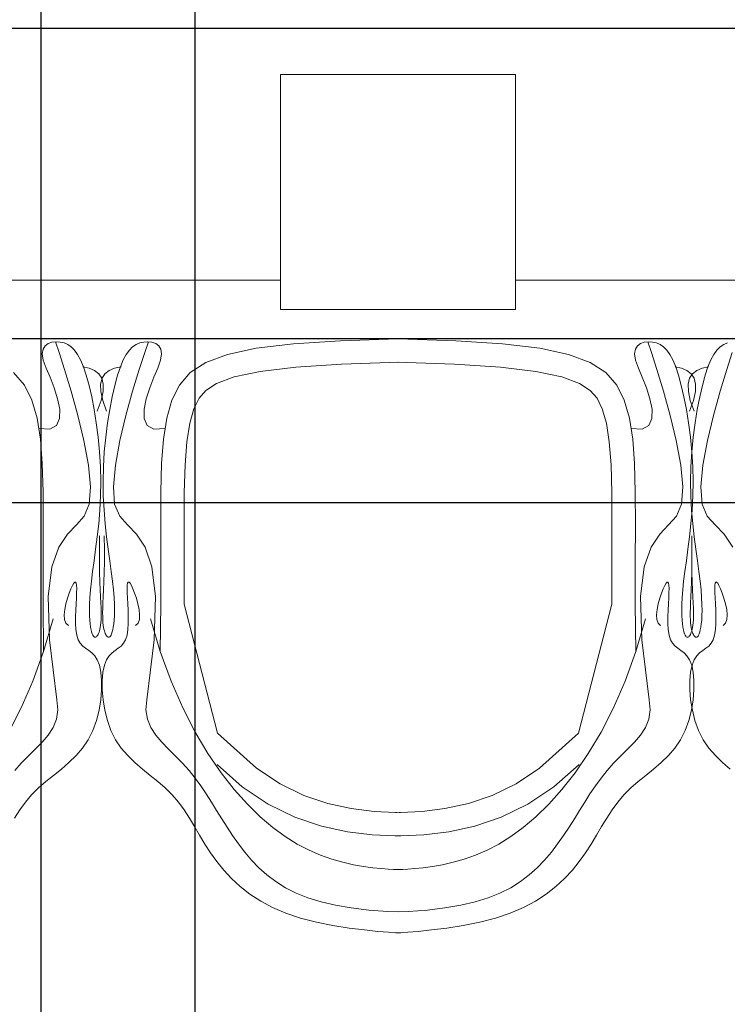
# Model space of a CAD drawing. Units: inches. Extents: x 1454 to 2136, y 626 to 1213.
# Tile 13 of 23: x 1654 to 1678, y 1062 to 1095. Entities that reach past the tile are written whole.
import ezdxf

# ---------------------------------------------------------------- set-up
doc = ezdxf.new("R2010")
doc.units = ezdxf.units.IN
doc.header["$MEASUREMENT"] = 0
for name, color, linetype, lineweight in [('A-ANNO-DIMS', 2, 'Continuous', 18), ('A-FURN-PATT', 252, 'Continuous', 13), ('conference', 41, 'Continuous', 18)]:
    doc.layers.add(name, color=color, linetype=linetype, lineweight=lineweight)
doc.styles.get("Standard").update_dxf_attribs({"font": 'arial.ttf'})
doc.dimstyles.get("Standard").update_dxf_attribs({"dimtxt": 4, "dimasz": 0.18, "dimexe": 0.18, "dimexo": 0.0625, "dimgap": 0.09, "dimtad": 0, "dimtih": 1, "dimtoh": 1, "dimdec": 0, "dimrnd": 6, "dimzin": 0, "dimdsep": 46, "dimlunit": 3, "dimtxsty": 'Standard', "dimcen": 0.09, "dimadec": 0, "dimazin": 0, "dimtfac": 1, "dimtdec": 0, "dimtofl": 0, "dimtmove": 0, "dimatfit": 3, "dimfxl": 1, "dimtolj": 1, "dimtzin": 0, "dimarcsym": 0})

# ---------------------------------------------------------------- blocks, each defined once
blk = doc.blocks.new('ОГ52_на12персон_стол2800х900')
for p, q in [((603.37, -395.68), (403.37, -395.68)), ((403.37, -395.68), (403.37, -595.68)), ((603.37, -595.68), (603.37, -395.68)), ((96.63, -570.68), (403.37, -570.68)), ((903.37, -570.68), (603.37, -570.68)), ((403.37, -595.68), (603.37, -595.68)), ((-1300, -620.68), (1300, -620.68)), ((201.27, -629.41), (203.03, -626.5)), ((203.03, -626.5), (205.63, -624.59)), ((205.63, -624.59), (208.81, -623.54)), ((208.81, -623.54), (212.3, -623.21)), ((214.94, -632.32), (211.87, -623.25)), ((212.3, -623.21), (215.83, -623.45)), ((215.83, -623.45), (219.16, -624.18)), ((219.16, -624.18), (222.29, -625.46)), ((222.29, -625.46), (225.24, -627.43)), ((225.24, -627.43), (228.02, -630.19)), ((277.5, -627.43), (274.71, -630.19)), ((280.44, -625.46), (277.5, -627.43)), ((283.57, -624.18), (280.44, -625.46)), ((286.91, -623.45), (283.57, -624.18)), ((290.43, -623.21), (286.91, -623.45)), ((287.79, -632.32), (290.86, -623.25)), ((293.92, -623.54), (290.43, -623.21)), ((297.1, -624.59), (293.92, -623.54)), ((299.71, -626.5), (297.1, -624.59)), ((301.46, -629.41), (299.71, -626.5)), ((382.76, -628.66), (414.4, -624.84)), ((414.4, -624.84), (454.25, -622.24)), ((454.25, -622.24), (503.37, -620.68)), ((552.48, -622.24), (503.37, -620.68)), ((592.33, -624.84), (552.48, -622.24)), ((623.97, -628.66), (592.33, -624.84)), ((705.28, -629.41), (707.03, -626.5)), ((707.03, -626.5), (709.63, -624.59)), ((709.63, -624.59), (712.81, -623.54)), ((712.81, -623.54), (716.3, -623.21)), ((718.94, -632.32), (715.88, -623.25)), ((716.3, -623.21), (719.83, -623.45)), ((719.83, -623.45), (723.17, -624.18)), ((723.17, -624.18), (726.3, -625.46)), ((726.3, -625.46), (729.24, -627.43)), ((729.24, -627.43), (732.02, -630.19)), ((777.5, -627.43), (774.71, -630.19)), ((780.44, -625.46), (777.5, -627.43)), ((783.57, -624.18), (780.44, -625.46)), ((200.64, -633.47), (201.27, -629.41)), ((201.4, -638.81), (200.64, -633.47)), ((219.64, -646.8), (214.94, -632.32)), ((228.02, -630.19), (230.67, -633.88)), ((230.67, -633.88), (233.21, -638.62)), ((272.06, -633.88), (269.53, -638.62)), ((274.71, -630.19), (272.06, -633.88)), ((283.1, -646.8), (287.79, -632.32)), ((301.33, -638.81), (302.09, -633.47)), ((302.09, -633.47), (301.46, -629.41)), ((339.9, -640.74), (358.28, -633.9)), ((358.28, -633.9), (382.76, -628.66)), ((648.45, -633.9), (623.97, -628.66)), ((666.83, -640.74), (648.45, -633.9)), ((704.65, -633.47), (705.28, -629.41)), ((705.41, -638.81), (704.65, -633.47)), ((723.64, -646.8), (718.94, -632.32)), ((732.02, -630.19), (734.67, -633.88)), ((734.67, -633.88), (737.21, -638.62)), ((772.06, -633.88), (769.53, -638.62)), ((774.71, -630.19), (772.06, -633.88)), ((783.1, -646.8), (787.79, -632.32)), ((203.83, -645.58), (201.4, -638.81)), ((233.21, -638.62), (235.66, -644.52)), ((240.55, -645.63), (235.08, -644.46)), ((235.66, -644.52), (238.05, -651.71)), ((262.18, -645.63), (267.66, -644.46)), ((267.07, -644.52), (264.68, -651.71)), ((269.53, -638.62), (267.07, -644.52)), ((298.9, -645.58), (301.33, -638.81)), ((326.58, -649.4), (339.9, -640.74)), ((386.06, -648.4), (416.25, -644.76)), ((416.25, -644.76), (455.22, -642.22)), ((455.22, -642.22), (504, -640.67)), ((551.51, -642.22), (502.73, -640.67)), ((590.48, -644.76), (551.51, -642.22)), ((620.68, -648.4), (590.48, -644.76)), ((680.15, -649.4), (666.83, -640.74)), ((707.83, -645.58), (705.41, -638.81)), ((737.21, -638.62), (739.66, -644.52)), ((744.55, -645.63), (739.08, -644.46)), ((739.66, -644.52), (742.06, -651.71)), ((762.18, -645.63), (767.66, -644.46)), ((767.07, -644.52), (764.68, -651.71)), ((769.53, -638.62), (767.07, -644.52)), ((185.47, -660.04), (176.15, -649.4)), ((203.83, -645.58), (207.2, -653.36)), ((207.2, -653.36), (210.7, -662.32)), ((225.22, -665.14), (219.64, -646.8)), ((238.05, -651.71), (240.4, -660.26)), ((245.15, -647.56), (240.55, -645.63)), ((248.77, -650.38), (245.15, -647.56)), ((251.26, -654.22), (248.77, -650.38)), ((251.47, -654.22), (253.96, -650.38)), ((253.96, -650.38), (257.58, -647.56)), ((257.58, -647.56), (262.18, -645.63)), ((264.68, -651.71), (262.34, -660.26)), ((277.51, -665.14), (283.1, -646.8)), ((295.53, -653.36), (292.03, -662.32)), ((298.9, -645.58), (295.53, -653.36)), ((317.26, -660.04), (326.58, -649.4)), ((348.95, -658.72), (363.89, -653.15)), ((363.89, -653.15), (386.06, -648.4)), ((642.84, -653.15), (620.68, -648.4)), ((657.78, -658.72), (642.84, -653.15)), ((689.48, -660.04), (680.15, -649.4)), ((707.83, -645.58), (711.21, -653.36)), ((711.21, -653.36), (714.71, -662.32)), ((729.22, -665.14), (723.64, -646.8)), ((742.06, -651.71), (744.4, -660.26)), ((749.16, -647.56), (744.55, -645.63)), ((752.77, -650.38), (749.16, -647.56)), ((751.47, -654.22), (753.96, -650.38)), ((755.26, -654.22), (752.77, -650.38)), ((753.96, -650.38), (757.58, -647.56)), ((757.58, -647.56), (762.18, -645.63)), ((764.68, -651.71), (762.34, -660.26)), ((777.51, -665.14), (783.1, -646.8)), ((191.85, -672.88), (185.47, -660.04)), ((240.4, -660.26), (242.64, -670.01)), ((250.24, -659.21), (251.47, -654.22)), ((250.39, -665.48), (250.24, -659.21)), ((252.49, -659.21), (251.26, -654.22)), ((252.34, -665.48), (252.49, -659.21)), ((262.34, -660.26), (260.09, -670.01)), ((310.88, -672.88), (317.26, -660.04)), ((339.8, -664.66), (348.95, -658.72)), ((666.94, -664.66), (657.78, -658.72)), ((695.85, -672.88), (689.48, -660.04)), ((744.4, -660.26), (746.64, -670.01)), ((750.24, -659.21), (751.47, -654.22)), ((750.39, -665.48), (750.24, -659.21)), ((756.5, -659.21), (755.26, -654.22)), ((756.34, -665.48), (756.5, -659.21)), ((762.34, -660.26), (760.09, -670.01)), ((210.7, -662.32), (213.67, -671.68)), ((230.95, -685.83), (225.22, -665.14)), ((242.64, -670.01), (244.72, -680.76)), ((252.06, -673.16), (250.39, -665.48)), ((250.67, -673.16), (252.34, -665.48)), ((260.09, -670.01), (258.01, -680.76)), ((271.78, -685.83), (277.51, -665.14)), ((292.03, -662.32), (289.06, -671.68)), ((334.02, -671.26), (339.8, -664.66)), ((672.72, -671.26), (666.94, -664.66)), ((714.71, -662.32), (717.68, -671.68)), ((734.96, -685.83), (729.22, -665.14)), ((746.64, -670.01), (748.73, -680.76)), ((752.06, -673.16), (750.39, -665.48)), ((754.67, -673.16), (756.34, -665.48)), ((760.09, -670.01), (758.01, -680.76)), ((771.78, -685.83), (777.51, -665.14)), ((196.21, -688.12), (191.85, -672.88)), ((213.67, -671.68), (215.46, -680.65)), ((247.35, -682.38), (250.67, -673.16)), ((255.38, -682.38), (252.06, -673.16)), ((289.06, -671.68), (287.28, -680.65)), ((306.53, -688.12), (310.88, -672.88)), ((329.61, -680.14), (334.02, -671.26)), ((677.13, -680.14), (672.72, -671.26)), ((700.21, -688.12), (695.85, -672.88)), ((717.68, -671.68), (719.46, -680.65)), ((751.36, -682.38), (754.67, -673.16)), ((755.38, -682.38), (752.06, -673.16)), ((215.46, -680.65), (215.4, -688.46)), ((236.09, -707.33), (230.95, -685.83)), ((244.72, -680.76), (246.58, -692.29)), ((258.01, -680.76), (256.16, -692.29)), ((266.64, -707.33), (271.78, -685.83)), ((287.28, -680.65), (287.33, -688.46)), ((326.1, -692.42), (329.61, -680.14)), ((680.64, -692.42), (677.13, -680.14)), ((719.46, -680.65), (719.4, -688.46)), ((740.09, -707.33), (734.96, -685.83)), ((748.73, -680.76), (750.58, -692.29)), ((758.01, -680.76), (756.16, -692.29)), ((766.64, -707.33), (771.78, -685.83)), ((199, -706.03), (196.21, -688.12)), ((212.84, -694.32), (207.13, -697.45)), ((215.4, -688.46), (212.84, -694.32)), ((246.58, -692.29), (248.14, -704.4)), ((256.16, -692.29), (254.59, -704.4)), ((287.33, -688.46), (289.89, -694.32)), ((289.89, -694.32), (295.6, -697.45)), ((303.73, -706.03), (306.53, -688.12)), ((323.61, -708.33), (326.1, -692.42)), ((683.12, -708.33), (680.64, -692.42)), ((703.01, -706.03), (700.21, -688.12)), ((716.84, -694.32), (711.13, -697.45)), ((719.4, -688.46), (716.84, -694.32)), ((750.58, -692.29), (752.14, -704.4)), ((756.16, -692.29), (754.59, -704.4)), ((207.13, -697.45), (197.6, -697.07)), ((295.6, -697.45), (305.13, -697.07)), ((711.13, -697.45), (701.61, -697.07)), ((200.57, -726.94), (199, -706.03)), ((239.89, -728.11), (236.09, -707.33)), ((248.14, -704.4), (249.35, -716.88)), ((254.59, -704.4), (253.38, -716.88)), ((262.84, -728.11), (266.64, -707.33)), ((302.16, -726.94), (303.73, -706.03)), ((322.14, -727.97), (323.61, -708.33)), ((684.6, -727.97), (683.12, -708.33)), ((704.57, -726.94), (703.01, -706.03)), ((743.89, -728.11), (740.09, -707.33)), ((752.14, -704.4), (753.35, -716.88)), ((754.59, -704.4), (753.38, -716.88)), ((762.84, -728.11), (766.64, -707.33)), ((249.35, -716.88), (250.14, -729.52)), ((253.38, -716.88), (252.59, -729.52)), ((753.38, -716.88), (752.59, -729.52)), ((753.35, -716.88), (754.14, -729.52)), ((201.25, -751.13), (200.57, -726.94)), ((241.62, -746.63), (239.89, -728.11)), ((261.12, -746.63), (262.84, -728.11)), ((301.49, -751.13), (302.16, -726.94)), ((321.48, -751.45), (322.14, -727.97)), ((685.25, -751.45), (684.6, -727.97)), ((705.25, -751.13), (704.57, -726.94)), ((745.62, -746.63), (743.89, -728.11)), ((761.12, -746.63), (762.84, -728.11)), ((250.14, -729.52), (250.45, -742.11)), ((252.59, -729.52), (252.29, -742.11)), ((752.59, -729.52), (752.29, -742.11)), ((754.14, -729.52), (754.45, -742.11)), ((250.45, -742.11), (250.23, -754.46)), ((252.29, -742.11), (252.5, -754.46)), ((752.29, -742.11), (752.5, -754.46)), ((754.45, -742.11), (754.24, -754.46)), ((201.36, -778.91), (201.25, -751.13)), ((240.52, -761.38), (241.62, -746.63)), ((262.21, -761.38), (261.12, -746.63)), ((301.37, -778.91), (301.49, -751.13)), ((321.37, -778.91), (321.48, -751.45)), ((685.37, -778.91), (685.25, -751.45)), ((705.37, -778.91), (705.25, -751.13)), ((744.53, -761.38), (745.62, -746.63)), ((762.21, -761.38), (761.12, -746.63)), ((236.21, -771.53), (240.52, -761.38)), ((250.23, -754.46), (249.58, -766.48)), ((252.5, -754.46), (253.15, -766.48)), ((266.53, -771.53), (262.21, -761.38)), ((740.21, -771.53), (744.53, -761.38)), ((752.5, -754.46), (753.15, -766.48)), ((754.24, -754.46), (753.59, -766.48)), ((766.53, -771.53), (762.21, -761.38)), ((249.58, -766.48), (248.6, -778.08)), ((253.15, -766.48), (254.14, -778.08)), ((753.59, -766.48), (752.6, -778.08)), ((753.15, -766.48), (754.14, -778.08)), ((201.25, -810.58), (201.36, -778.91)), ((221.98, -787.04), (229.6, -779.15)), ((229.6, -779.15), (236.21, -771.53)), ((248.6, -778.08), (247.38, -789.18)), ((254.14, -778.08), (255.35, -789.18)), ((273.13, -779.15), (266.53, -771.53)), ((280.75, -787.04), (273.13, -779.15)), ((301.48, -810.58), (301.37, -778.91)), ((321.48, -810.54), (321.37, -778.91)), ((685.26, -810.54), (685.37, -778.91)), ((705.26, -810.58), (705.37, -778.91)), ((725.99, -787.04), (733.61, -779.15)), ((733.61, -779.15), (740.21, -771.53)), ((752.6, -778.08), (751.38, -789.18)), ((754.14, -778.08), (755.35, -789.18)), ((773.13, -779.15), (766.53, -771.53)), ((780.75, -787.04), (773.13, -779.15)), ((214.62, -797.97), (221.98, -787.04)), ((288.11, -797.97), (280.75, -787.04)), ((718.62, -797.97), (725.99, -787.04)), ((788.11, -797.97), (780.75, -787.04)), ((247.38, -789.18), (246.04, -799.7)), ((249.27, -800.21), (249.41, -788.46)), ((253.46, -800.21), (253.32, -788.46)), ((255.35, -789.18), (256.69, -799.7)), ((751.38, -789.18), (750.05, -799.7)), ((753.27, -800.21), (753.41, -788.46)), ((753.46, -800.21), (753.32, -788.46)), ((755.35, -789.18), (756.69, -799.7)), ((208.78, -814.73), (214.62, -797.97)), ((246.04, -799.7), (244.69, -809.56)), ((249.29, -810.55), (249.27, -800.21)), ((253.45, -810.55), (253.46, -800.21)), ((256.69, -799.7), (258.04, -809.56)), ((293.95, -814.73), (288.11, -797.97)), ((712.78, -814.73), (718.62, -797.97)), ((750.05, -799.7), (748.69, -809.56)), ((753.29, -810.55), (753.27, -800.21)), ((753.45, -810.55), (753.46, -800.21)), ((756.69, -799.7), (758.04, -809.56)), ((201.25, -846.44), (201.25, -810.58)), ((244.69, -809.56), (243.43, -818.69)), ((249.43, -819.6), (249.29, -810.55)), ((253.3, -819.6), (253.45, -810.55)), ((258.04, -809.56), (259.3, -818.69)), ((301.48, -846.44), (301.48, -810.58)), ((321.48, -846.55), (321.48, -810.54)), ((685.26, -846.55), (685.26, -810.54)), ((705.26, -846.44), (705.26, -810.58)), ((748.69, -809.56), (747.43, -818.69)), ((753.43, -819.6), (753.29, -810.55)), ((753.3, -819.6), (753.45, -810.55)), ((758.04, -809.56), (759.3, -818.69)), ((205.74, -840.11), (208.78, -814.73)), ((243.43, -818.69), (242.36, -826.99)), ((249.65, -827.5), (249.43, -819.6)), ((253.08, -827.5), (253.3, -819.6)), ((259.3, -818.69), (260.37, -826.99)), ((296.99, -840.11), (293.95, -814.73)), ((709.75, -840.11), (712.78, -814.73)), ((747.43, -818.69), (746.37, -826.99)), ((753.08, -827.5), (753.3, -819.6)), ((753.66, -827.5), (753.43, -819.6)), ((759.3, -818.69), (760.37, -826.99)), ((226.32, -830.57), (227.4, -828.7)), ((227.4, -828.7), (228.29, -827.76)), ((228.29, -827.76), (228.98, -827.75)), ((228.98, -827.75), (229.48, -828.65)), ((229.48, -828.65), (229.79, -830.45)), ((242.36, -826.99), (241.58, -834.42)), ((249.92, -834.35), (249.65, -827.5)), ((252.81, -834.35), (253.08, -827.5)), ((260.37, -826.99), (261.16, -834.42)), ((273.25, -828.65), (272.94, -830.45)), ((273.75, -827.75), (273.25, -828.65)), ((274.44, -827.76), (273.75, -827.75)), ((275.33, -828.7), (274.44, -827.76)), ((276.41, -830.57), (275.33, -828.7)), ((730.32, -830.57), (731.41, -828.7)), ((731.41, -828.7), (732.29, -827.76)), ((732.29, -827.76), (732.98, -827.75)), ((732.98, -827.75), (733.48, -828.65)), ((733.48, -828.65), (733.79, -830.45)), ((746.37, -826.99), (745.58, -834.42)), ((752.81, -834.35), (753.08, -827.5)), ((753.93, -834.35), (753.66, -827.5)), ((760.37, -826.99), (761.16, -834.42)), ((773.25, -828.65), (772.94, -830.45)), ((773.75, -827.75), (773.25, -828.65)), ((774.44, -827.76), (773.75, -827.75)), ((775.33, -828.7), (774.44, -827.76)), ((776.41, -830.57), (775.33, -828.7)), ((222.07, -841.47), (223.56, -837.1)), ((223.56, -837.1), (225.03, -833.39)), ((225.03, -833.39), (226.32, -830.57)), ((229.87, -836.73), (229.66, -841.16)), ((229.79, -830.45), (229.92, -833.15)), ((229.92, -833.15), (229.87, -836.73)), ((241.58, -834.42), (241.06, -841)), ((250.2, -840.27), (249.92, -834.35)), ((252.53, -840.27), (252.81, -834.35)), ((261.16, -834.42), (261.67, -841)), ((272.94, -830.45), (272.81, -833.15)), ((272.81, -833.15), (272.87, -836.73)), ((272.87, -836.73), (273.08, -841.16)), ((277.7, -833.39), (276.41, -830.57)), ((279.17, -837.1), (277.7, -833.39)), ((280.66, -841.47), (279.17, -837.1)), ((726.07, -841.47), (727.56, -837.1)), ((727.56, -837.1), (729.03, -833.39)), ((729.03, -833.39), (730.32, -830.57)), ((733.87, -836.73), (733.66, -841.16)), ((733.79, -830.45), (733.92, -833.15)), ((733.92, -833.15), (733.87, -836.73)), ((745.58, -834.42), (745.06, -841)), ((752.53, -840.27), (752.81, -834.35)), ((754.21, -840.27), (753.93, -834.35)), ((761.16, -834.42), (761.67, -841)), ((772.94, -830.45), (772.81, -833.15)), ((772.81, -833.15), (772.87, -836.73)), ((772.87, -836.73), (773.08, -841.16)), ((777.7, -833.39), (776.41, -830.57)), ((779.17, -837.1), (777.7, -833.39)), ((780.66, -841.47), (779.17, -837.1)), ((201.7, -886.8), (201.25, -846.44)), ((206.77, -876.9), (205.74, -840.11)), ((219.73, -850.99), (220.73, -846.2)), ((220.73, -846.2), (222.07, -841.47)), ((229.36, -846.22), (229.09, -851.69)), ((229.66, -841.16), (229.36, -846.22)), ((241.06, -841), (240.78, -846.8)), ((250.46, -845.39), (250.2, -840.27)), ((250.64, -849.83), (250.46, -845.39)), ((252.09, -849.83), (252.28, -845.39)), ((252.28, -845.39), (252.53, -840.27)), ((261.67, -841), (261.96, -846.8)), ((273.08, -841.16), (273.37, -846.22)), ((273.37, -846.22), (273.65, -851.69)), ((282, -846.2), (280.66, -841.47)), ((283, -850.99), (282, -846.2)), ((295.96, -876.9), (296.99, -840.11)), ((301.03, -886.8), (301.48, -846.44)), ((349.76, -956.38), (321.48, -846.55)), ((656.98, -956.38), (685.26, -846.55)), ((705.7, -886.8), (705.26, -846.44)), ((710.78, -876.9), (709.75, -840.11)), ((723.74, -850.99), (724.74, -846.2)), ((724.74, -846.2), (726.07, -841.47)), ((733.37, -846.22), (733.09, -851.69)), ((733.66, -841.16), (733.37, -846.22)), ((745.06, -841), (744.78, -846.8)), ((752.09, -849.83), (752.28, -845.39)), ((752.28, -845.39), (752.53, -840.27)), ((754.46, -845.39), (754.21, -840.27)), ((754.65, -849.83), (754.46, -845.39)), ((761.67, -841), (761.96, -846.8)), ((773.08, -841.16), (773.37, -846.22)), ((773.37, -846.22), (773.65, -851.69)), ((782, -846.2), (780.66, -841.47)), ((783, -850.99), (782, -846.2)), ((219.26, -855.54), (219.73, -850.99)), ((229.09, -851.69), (228.91, -857.33)), ((240.78, -846.8), (240.7, -851.87)), ((240.7, -851.87), (240.79, -856.27)), ((250.73, -853.68), (250.64, -849.83)), ((250.72, -857.02), (250.73, -853.68)), ((252, -853.68), (252.09, -849.83)), ((252.01, -857.02), (252, -853.68)), ((262.04, -851.87), (261.95, -856.27)), ((261.96, -846.8), (262.04, -851.87)), ((273.65, -851.69), (273.82, -857.33)), ((283.47, -855.54), (283, -850.99)), ((723.26, -855.54), (723.74, -850.99)), ((733.09, -851.69), (732.92, -857.33)), ((744.78, -846.8), (744.7, -851.87)), ((744.7, -851.87), (744.79, -856.27)), ((752, -853.68), (752.09, -849.83)), ((752.01, -857.02), (752, -853.68)), ((754.73, -853.68), (754.65, -849.83)), ((754.73, -857.02), (754.73, -853.68)), ((762.04, -851.87), (761.95, -856.27)), ((761.96, -846.8), (762.04, -851.87)), ((773.65, -851.69), (773.82, -857.33)), ((783.47, -855.54), (783, -850.99)), ((210, -858.96), (201.71, -886.79)), ((219.49, -859.55), (219.26, -855.54)), ((220.61, -862.74), (219.49, -859.55)), ((222.8, -864.79), (220.61, -862.74)), ((228.91, -857.33), (228.94, -862.89)), ((228.94, -862.89), (229.27, -868.16)), ((240.79, -856.27), (241.01, -860.06)), ((241.01, -860.06), (241.34, -863.29)), ((241.34, -863.29), (241.73, -866.03)), ((250.24, -864.48), (250.47, -862.37)), ((250.47, -862.37), (250.63, -859.89)), ((250.63, -859.89), (250.72, -857.02)), ((252.1, -859.89), (252.01, -857.02)), ((252.26, -862.37), (252.1, -859.89)), ((252.49, -864.48), (252.26, -862.37)), ((261.4, -863.29), (261, -866.03)), ((261.72, -860.06), (261.4, -863.29)), ((261.95, -856.27), (261.72, -860.06)), ((273.79, -862.89), (273.47, -868.16)), ((273.82, -857.33), (273.79, -862.89)), ((279.93, -864.79), (282.12, -862.74)), ((282.12, -862.74), (283.24, -859.55)), ((283.24, -859.55), (283.47, -855.54)), ((292.73, -858.96), (301.02, -886.79)), ((714, -858.96), (705.72, -886.79)), ((723.49, -859.55), (723.26, -855.54)), ((724.61, -862.74), (723.49, -859.55)), ((726.8, -864.79), (724.61, -862.74)), ((732.92, -857.33), (732.95, -862.89)), ((732.95, -862.89), (733.27, -868.16)), ((744.79, -856.27), (745.01, -860.06)), ((745.01, -860.06), (745.34, -863.29)), ((745.34, -863.29), (745.73, -866.03)), ((752.1, -859.89), (752.01, -857.02)), ((752.26, -862.37), (752.1, -859.89)), ((752.49, -864.48), (752.26, -862.37)), ((754.25, -864.48), (754.47, -862.37)), ((754.47, -862.37), (754.64, -859.89)), ((754.64, -859.89), (754.73, -857.02)), ((761.4, -863.29), (761, -866.03)), ((761.72, -860.06), (761.4, -863.29)), ((761.95, -856.27), (761.72, -860.06)), ((773.79, -862.89), (773.47, -868.16)), ((773.82, -857.33), (773.79, -862.89)), ((779.93, -864.79), (782.12, -862.74)), ((782.12, -862.74), (783.24, -859.55)), ((783.24, -859.55), (783.47, -855.54)), ((229.27, -868.16), (229.98, -872.89)), ((241.73, -866.03), (242.17, -868.32)), ((242.17, -868.32), (242.63, -870.2)), ((242.63, -870.2), (243.11, -871.7)), ((243.11, -871.7), (243.62, -872.86)), ((248.07, -872.49), (248.49, -871.56)), ((248.49, -871.56), (248.9, -870.47)), ((248.9, -870.47), (249.28, -869.25)), ((249.28, -869.25), (249.64, -867.87)), ((249.64, -867.87), (249.96, -866.3)), ((249.96, -866.3), (250.24, -864.48)), ((252.77, -866.3), (252.49, -864.48)), ((253.09, -867.87), (252.77, -866.3)), ((253.45, -869.25), (253.09, -867.87)), ((253.83, -870.47), (253.45, -869.25)), ((254.24, -871.56), (253.83, -870.47)), ((254.66, -872.49), (254.24, -871.56)), ((259.62, -871.7), (259.11, -872.86)), ((260.1, -870.2), (259.62, -871.7)), ((260.57, -868.32), (260.1, -870.2)), ((261, -866.03), (260.57, -868.32)), ((273.47, -868.16), (272.75, -872.89)), ((733.27, -868.16), (733.98, -872.89)), ((745.73, -866.03), (746.17, -868.32)), ((746.17, -868.32), (746.63, -870.2)), ((746.63, -870.2), (747.12, -871.7)), ((747.12, -871.7), (747.62, -872.86)), ((752.07, -872.49), (752.5, -871.56)), ((752.77, -866.3), (752.49, -864.48)), ((752.5, -871.56), (752.9, -870.47)), ((753.09, -867.87), (752.77, -866.3)), ((752.9, -870.47), (753.28, -869.25)), ((753.45, -869.25), (753.09, -867.87)), ((753.28, -869.25), (753.64, -867.87)), ((753.83, -870.47), (753.45, -869.25)), ((753.64, -867.87), (753.97, -866.3)), ((754.24, -871.56), (753.83, -870.47)), ((753.97, -866.3), (754.25, -864.48)), ((754.66, -872.49), (754.24, -871.56)), ((759.62, -871.7), (759.11, -872.86)), ((760.1, -870.2), (759.62, -871.7)), ((760.57, -868.32), (760.1, -870.2)), ((761, -866.03), (760.57, -868.32)), ((773.47, -868.16), (772.75, -872.89)), ((213.14, -927.87), (206.77, -876.9)), ((229.98, -872.89), (231.17, -876.84)), ((231.17, -876.84), (232.9, -879.87)), ((232.9, -879.87), (235.06, -882.2)), ((243.62, -872.86), (244.13, -873.71)), ((244.13, -873.71), (244.66, -874.27)), ((244.66, -874.27), (245.18, -874.59)), ((245.18, -874.59), (245.69, -874.69)), ((245.69, -874.69), (246.2, -874.6)), ((246.2, -874.6), (246.69, -874.32)), ((246.69, -874.32), (247.16, -873.88)), ((247.16, -873.88), (247.63, -873.27)), ((247.63, -873.27), (248.07, -872.49)), ((255.11, -873.27), (254.66, -872.49)), ((255.57, -873.88), (255.11, -873.27)), ((256.04, -874.32), (255.57, -873.88)), ((256.54, -874.6), (256.04, -874.32)), ((257.04, -874.69), (256.54, -874.6)), ((257.56, -874.59), (257.04, -874.69)), ((258.08, -874.27), (257.56, -874.59)), ((258.6, -873.71), (258.08, -874.27)), ((259.11, -872.86), (258.6, -873.71)), ((269.83, -879.87), (267.67, -882.2)), ((271.56, -876.84), (269.83, -879.87)), ((272.75, -872.89), (271.56, -876.84)), ((289.59, -927.87), (295.96, -876.9)), ((717.15, -927.87), (710.78, -876.9)), ((733.98, -872.89), (735.17, -876.84)), ((735.17, -876.84), (736.9, -879.87)), ((736.9, -879.87), (739.07, -882.2)), ((747.62, -872.86), (748.14, -873.71)), ((748.14, -873.71), (748.66, -874.27)), ((748.66, -874.27), (749.18, -874.59)), ((749.18, -874.59), (749.7, -874.69)), ((749.7, -874.69), (750.2, -874.6)), ((750.2, -874.6), (750.69, -874.32)), ((750.69, -874.32), (751.17, -873.88)), ((751.17, -873.88), (751.63, -873.27)), ((751.63, -873.27), (752.07, -872.49)), ((755.11, -873.27), (754.66, -872.49)), ((755.57, -873.88), (755.11, -873.27)), ((756.04, -874.32), (755.57, -873.88)), ((756.54, -874.6), (756.04, -874.32)), ((757.04, -874.69), (756.54, -874.6)), ((757.56, -874.59), (757.04, -874.69)), ((758.08, -874.27), (757.56, -874.59)), ((758.6, -873.71), (758.08, -874.27)), ((759.11, -872.86), (758.6, -873.71)), ((769.83, -879.87), (767.67, -882.2)), ((771.56, -876.84), (769.83, -879.87)), ((772.75, -872.89), (771.56, -876.84)), ((201.71, -886.79), (192.52, -912.08)), ((235.06, -882.2), (237.52, -884.13)), ((237.52, -884.13), (240.12, -885.97)), ((240.12, -885.97), (242.74, -888.03)), ((242.74, -888.03), (245.22, -890.62)), ((260, -888.03), (257.52, -890.62)), ((262.61, -885.97), (260, -888.03)), ((265.22, -884.13), (262.61, -885.97)), ((267.67, -882.2), (265.22, -884.13)), ((301.02, -886.79), (310.21, -912.08)), ((705.72, -886.79), (696.52, -912.08)), ((739.07, -882.2), (741.52, -884.13)), ((741.52, -884.13), (744.12, -885.97)), ((744.12, -885.97), (746.74, -888.03)), ((746.74, -888.03), (749.22, -890.62)), ((760, -888.03), (757.52, -890.62)), ((762.61, -885.97), (760, -888.03)), ((765.22, -884.13), (762.61, -885.97)), ((767.67, -882.2), (765.22, -884.13)), ((245.22, -890.62), (247.42, -894.03)), ((247.42, -894.03), (249.21, -898.59)), ((255.31, -894.03), (253.52, -898.59)), ((257.52, -890.62), (255.31, -894.03)), ((749.22, -890.62), (751.43, -894.03)), ((751.43, -894.03), (753.22, -898.59)), ((755.31, -894.03), (753.52, -898.59)), ((757.52, -890.62), (755.31, -894.03)), ((249.21, -898.59), (250.46, -904.49)), ((250.46, -904.49), (251.1, -911.55)), ((252.27, -904.49), (251.63, -911.55)), ((253.52, -898.59), (252.27, -904.49)), ((752.27, -904.49), (751.63, -911.55)), ((753.52, -898.59), (752.27, -904.49)), ((753.22, -898.59), (754.46, -904.49)), ((754.46, -904.49), (755.11, -911.55)), ((192.52, -912.08), (182.59, -934.93)), ((251.1, -911.55), (251.1, -919.48)), ((251.63, -911.55), (251.63, -919.48)), ((310.21, -912.08), (320.14, -934.93)), ((696.52, -912.08), (686.59, -934.93)), ((751.63, -911.55), (751.63, -919.48)), ((755.11, -911.55), (755.1, -919.48)), ((251.1, -919.48), (250.4, -927.99)), ((251.63, -919.48), (252.33, -927.99)), ((751.63, -919.48), (752.33, -927.99)), ((755.1, -919.48), (754.4, -927.99)), ((213.14, -927.87), (213.95, -936.53)), ((250.4, -927.99), (248.96, -936.78)), ((252.33, -927.99), (253.78, -936.78)), ((289.59, -927.87), (288.79, -936.53)), ((717.15, -927.87), (717.95, -936.53)), ((752.33, -927.99), (753.78, -936.78)), ((754.4, -927.99), (752.96, -936.78)), ((182.59, -934.93), (172.08, -955.46)), ((213.95, -936.53), (212.72, -944.33)), ((248.96, -936.78), (246.73, -945.57)), ((253.78, -936.78), (256, -945.57)), ((288.79, -936.53), (290.01, -944.33)), ((320.14, -934.93), (330.65, -955.46)), ((686.59, -934.93), (676.08, -955.46)), ((717.95, -936.53), (716.73, -944.33)), ((752.96, -936.78), (750.73, -945.57)), ((753.78, -936.78), (756, -945.57)), ((212.72, -944.33), (209.83, -951.42)), ((246.73, -945.57), (243.67, -954.07)), ((256, -945.57), (259.07, -954.07)), ((290.01, -944.33), (292.9, -951.42)), ((716.73, -944.33), (713.84, -951.42)), ((750.73, -945.57), (747.67, -954.07)), ((756, -945.57), (759.07, -954.07)), ((209.83, -951.42), (205.63, -957.97)), ((243.67, -954.07), (239.73, -961.98)), ((259.07, -954.07), (263.01, -961.98)), ((292.9, -951.42), (297.11, -957.97)), ((330.65, -955.46), (341.58, -973.79)), ((676.08, -955.46), (665.16, -973.79)), ((713.84, -951.42), (709.63, -957.97)), ((747.67, -954.07), (743.73, -961.98)), ((759.07, -954.07), (763.01, -961.98)), ((205.63, -957.97), (200.46, -964.14)), ((239.73, -961.98), (234.9, -969.1)), ((263.01, -961.98), (267.83, -969.1)), ((297.11, -957.97), (302.27, -964.14)), ((349.76, -956.38), (383.04, -986.28)), ((656.98, -956.38), (623.7, -986.28)), ((709.63, -957.97), (704.47, -964.14)), ((743.73, -961.98), (738.91, -969.1)), ((763.01, -961.98), (767.83, -969.1)), ((194.7, -970.09), (188.68, -975.98)), ((200.46, -964.14), (194.7, -970.09)), ((234.9, -969.1), (229.35, -975.52)), ((267.83, -969.1), (273.38, -975.52)), ((302.27, -964.14), (308.04, -970.09)), ((308.04, -970.09), (314.05, -975.98)), ((698.7, -970.09), (692.68, -975.98)), ((704.47, -964.14), (698.7, -970.09)), ((738.91, -969.1), (733.35, -975.52)), ((767.83, -969.1), (773.38, -975.52)), ((188.68, -975.98), (182.77, -981.97)), ((229.35, -975.52), (223.26, -981.41)), ((273.38, -975.52), (279.47, -981.41)), ((314.05, -975.98), (319.96, -981.97)), ((341.58, -973.79), (352.75, -990.05)), ((665.16, -973.79), (653.98, -990.05)), ((692.68, -975.98), (686.78, -981.97)), ((733.35, -975.52), (727.26, -981.41)), ((773.38, -975.52), (779.47, -981.41)), ((182.77, -981.97), (177.25, -988.18)), ((216.83, -986.94), (210.24, -992.27)), ((223.26, -981.41), (216.83, -986.94)), ((279.47, -981.41), (285.91, -986.94)), ((285.91, -986.94), (292.49, -992.27)), ((319.96, -981.97), (325.48, -988.18)), ((325.48, -988.18), (330.62, -994.63)), ((349.41, -982.95), (370.75, -1002.12)), ((383.04, -986.28), (402.91, -999.52)), ((623.7, -986.28), (603.83, -999.52)), ((657.33, -982.95), (635.99, -1002.12)), ((681.26, -988.18), (676.12, -994.63)), ((686.78, -981.97), (681.26, -988.18)), ((720.83, -986.94), (714.25, -992.27)), ((727.26, -981.41), (720.83, -986.94)), ((779.47, -981.41), (785.91, -986.94)), ((210.24, -992.27), (203.71, -997.59)), ((292.49, -992.27), (299.02, -997.59)), ((330.62, -994.63), (335.45, -1001.27)), ((352.75, -990.05), (364.01, -1004.34)), ((653.98, -990.05), (642.73, -1004.34)), ((676.12, -994.63), (671.28, -1001.27)), ((714.25, -992.27), (707.71, -997.59)), ((197.41, -1003.05), (191.55, -1008.83)), ((203.71, -997.59), (197.41, -1003.05)), ((299.02, -997.59), (305.32, -1003.05)), ((305.32, -1003.05), (311.18, -1008.83)), ((335.45, -1001.27), (340.06, -1008.08)), ((364.01, -1004.34), (375.19, -1016.78)), ((370.75, -1002.12), (392.96, -1016.92)), ((402.91, -999.52), (423.17, -1009.34)), ((603.83, -999.52), (583.56, -1009.34)), ((635.99, -1002.12), (613.78, -1016.92)), ((642.73, -1004.34), (631.55, -1016.78)), ((671.28, -1001.27), (666.67, -1008.08)), ((701.42, -1003.05), (695.56, -1008.83)), ((707.71, -997.59), (701.42, -1003.05)), ((191.55, -1008.83), (186.26, -1015.06)), ((311.18, -1008.83), (316.47, -1015.06)), ((340.06, -1008.08), (344.54, -1015.03)), ((423.17, -1009.34), (443.52, -1016.23)), ((583.56, -1009.34), (563.22, -1016.23)), ((666.67, -1008.08), (662.2, -1015.03)), ((695.56, -1008.83), (690.26, -1015.06)), ((181.44, -1021.69), (176.93, -1028.66)), ((186.26, -1015.06), (181.44, -1021.69)), ((316.47, -1015.06), (321.29, -1021.69)), ((321.29, -1021.69), (325.8, -1028.66)), ((344.54, -1015.03), (348.95, -1022.08)), ((348.95, -1022.08), (353.38, -1029.21)), ((375.19, -1016.78), (386.15, -1027.51)), ((392.96, -1016.92), (415.58, -1027.88)), ((443.52, -1016.23), (463.59, -1020.64)), ((463.59, -1020.64), (482.99, -1023.02)), ((543.14, -1020.64), (523.75, -1023.02)), ((563.22, -1016.23), (543.14, -1020.64)), ((613.78, -1016.92), (591.16, -1027.88)), ((631.55, -1016.78), (620.58, -1027.51)), ((657.79, -1022.08), (653.36, -1029.21)), ((662.2, -1015.03), (657.79, -1022.08)), ((685.44, -1021.69), (680.94, -1028.66)), ((690.26, -1015.06), (685.44, -1021.69)), ((325.8, -1028.66), (330.15, -1035.88)), ((353.38, -1029.21), (357.9, -1036.39)), ((386.15, -1027.51), (396.87, -1036.65)), ((415.58, -1027.88), (438.15, -1035.52)), ((482.99, -1023.02), (501.26, -1023.82)), ((501.26, -1023.82), (502.98, -1023.78)), ((505.48, -1023.82), (503.76, -1023.78)), ((523.75, -1023.02), (505.48, -1023.82)), ((591.16, -1027.88), (568.59, -1035.52)), ((620.58, -1027.51), (609.86, -1036.65)), ((653.36, -1029.21), (648.83, -1036.39)), ((680.94, -1028.66), (676.58, -1035.88)), ((330.15, -1035.88), (334.5, -1043.27)), ((357.9, -1036.39), (362.61, -1043.58)), ((396.87, -1036.65), (407.36, -1044.36)), ((438.15, -1035.52), (460.22, -1040.38)), ((568.59, -1035.52), (546.52, -1040.38)), ((609.86, -1036.65), (599.37, -1044.36)), ((648.83, -1036.39), (644.13, -1043.58)), ((676.58, -1035.88), (672.23, -1043.27)), ((334.5, -1043.27), (339.01, -1050.76)), ((362.61, -1043.58), (367.57, -1050.71)), ((407.36, -1044.36), (417.61, -1050.77)), ((460.22, -1040.38), (481.33, -1042.97)), ((481.33, -1042.97), (501.02, -1043.83)), ((501.02, -1043.83), (503.37, -1043.78)), ((505.72, -1043.83), (503.37, -1043.78)), ((525.41, -1042.97), (505.72, -1043.83)), ((546.52, -1040.38), (525.41, -1042.97)), ((599.37, -1044.36), (589.12, -1050.77)), ((644.13, -1043.58), (639.16, -1050.71)), ((672.23, -1043.27), (667.73, -1050.76)), ((339.01, -1050.76), (343.83, -1058.27)), ((367.57, -1050.71), (372.88, -1057.7)), ((417.61, -1050.77), (427.64, -1056.02)), ((427.64, -1056.02), (437.43, -1060.26)), ((579.1, -1056.02), (569.31, -1060.26)), ((589.12, -1050.77), (579.1, -1056.02)), ((639.16, -1050.71), (633.85, -1057.7)), ((667.73, -1050.76), (662.91, -1058.27)), ((343.83, -1058.27), (349.12, -1065.72)), ((372.88, -1057.7), (378.62, -1064.48)), ((378.62, -1064.48), (384.87, -1070.97)), ((437.43, -1060.26), (447, -1063.63)), ((447, -1063.63), (456.35, -1066.28)), ((559.74, -1063.63), (550.39, -1066.28)), ((569.31, -1060.26), (559.74, -1063.63)), ((628.11, -1064.48), (621.86, -1070.97)), ((633.85, -1057.7), (628.11, -1064.48)), ((662.91, -1058.27), (657.61, -1065.72)), ((349.12, -1065.72), (355.03, -1073.02)), ((384.87, -1070.97), (391.71, -1077.1)), ((456.35, -1066.28), (465.43, -1068.34)), ((465.43, -1068.34), (474.07, -1069.88)), ((474.07, -1069.88), (482.02, -1070.98)), ((482.02, -1070.98), (489.06, -1071.72)), ((489.06, -1071.72), (494.94, -1072.17)), ((494.94, -1072.17), (499.45, -1072.4)), ((499.45, -1072.4), (502.33, -1072.49)), ((502.33, -1072.49), (503.37, -1072.5)), ((504.4, -1072.49), (503.37, -1072.5)), ((507.29, -1072.4), (504.4, -1072.49)), ((511.79, -1072.17), (507.29, -1072.4)), ((517.68, -1071.72), (511.79, -1072.17)), ((524.71, -1070.98), (517.68, -1071.72)), ((532.66, -1069.88), (524.71, -1070.98)), ((541.3, -1068.34), (532.66, -1069.88)), ((550.39, -1066.28), (541.3, -1068.34)), ((621.86, -1070.97), (615.02, -1077.1)), ((657.61, -1065.72), (651.71, -1073.02)), ((355.03, -1073.02), (361.64, -1080.11)), ((361.64, -1080.11), (369.03, -1086.91)), ((391.71, -1077.1), (399.23, -1082.79)), ((615.02, -1077.1), (607.5, -1082.79)), ((645.1, -1080.11), (637.71, -1086.91)), ((651.71, -1073.02), (645.1, -1080.11)), ((369.03, -1086.91), (377.28, -1093.35)), ((399.23, -1082.79), (407.51, -1087.97)), ((407.51, -1087.97), (416.64, -1092.56)), ((599.22, -1087.97), (590.1, -1092.56)), ((607.5, -1082.79), (599.22, -1087.97)), ((637.71, -1086.91), (629.46, -1093.35)), ((377.28, -1093.35), (386.46, -1099.33)), ((416.64, -1092.56), (426.71, -1096.58)), ((426.71, -1096.58), (437.82, -1100.01)), ((580.03, -1096.58), (568.92, -1100.01)), ((590.1, -1092.56), (580.03, -1096.58)), ((629.46, -1093.35), (620.28, -1099.33)), ((386.46, -1099.33), (396.65, -1104.8)), ((396.65, -1104.8), (407.92, -1109.67)), ((437.82, -1100.01), (450.08, -1102.88)), ((450.08, -1102.88), (463.59, -1105.18)), ((463.59, -1105.18), (478.44, -1106.93)), ((543.15, -1105.18), (528.29, -1106.93)), ((556.66, -1102.88), (543.15, -1105.18)), ((568.92, -1100.01), (556.66, -1102.88)), ((610.09, -1104.8), (598.81, -1109.67)), ((620.28, -1099.33), (610.09, -1104.8)), ((407.92, -1109.67), (420.36, -1113.86)), ((420.36, -1113.86), (433.9, -1117.34)), ((478.44, -1106.93), (494.75, -1108.13)), ((494.75, -1108.13), (503.37, -1108.44)), ((511.98, -1108.13), (503.37, -1108.44)), ((528.29, -1106.93), (511.98, -1108.13)), ((586.38, -1113.86), (572.83, -1117.34)), ((598.81, -1109.67), (586.38, -1113.86)), ((433.9, -1117.34), (447.97, -1120.12)), ((447.97, -1120.12), (461.84, -1122.3)), ((461.84, -1122.3), (474.82, -1123.93)), ((544.89, -1122.3), (531.92, -1123.93)), ((558.77, -1120.12), (544.89, -1122.3)), ((572.83, -1117.34), (558.77, -1120.12)), ((474.82, -1123.93), (486.17, -1125.08)), ((486.17, -1125.08), (495.19, -1125.82)), ((495.19, -1125.82), (501.16, -1126.21)), ((501.16, -1126.21), (503.37, -1126.33)), ((505.58, -1126.21), (503.37, -1126.33)), ((511.55, -1125.82), (505.58, -1126.21)), ((520.57, -1125.08), (511.55, -1125.82)), ((531.92, -1123.93), (520.57, -1125.08))]:
    blk.add_line(p, q)
blk = doc.blocks.new('*D33')
at = {"layer": 'A-ANNO-DIMS', "color": 0, "lineweight": -2, "transparency": 16777216}
for p, q in [((2032.494, 1126.282), (1462.374, 1126.282)), ((1462.554, 1126.102), (1462.554, 1056.381)), ((1462.554, 982.462), (1462.554, 1052.184)), ((2032.494, 982.282), (1462.374, 982.282))]:
    blk.add_line(p, q, dxfattribs=at)
at = {"layer": 'A-ANNO-DIMS', "color": 0, "transparency": 16777216}
for points in [[(1462.524, 1126.102), (1462.584, 1126.102), (1462.554, 1126.282)], [(1462.524, 982.462), (1462.584, 982.462), (1462.554, 982.282)]]:
    blk.add_solid(points, dxfattribs=at)
at = {"layer": 'Defpoints', "color": 0, "transparency": 16777216}
for p in [(1462.554, 1126.282), (2032.556, 1126.282), (2032.556, 982.282)]:
    blk.add_point(p, dxfattribs=at)
at = {"layer": 'A-ANNO-DIMS', "color": 0, "transparency": 16777216, "insert": (1462.554, 1054.282), "char_height": 4, "attachment_point": 5}
blk.add_mtext('\\A1;144', dxfattribs=at)
blk = doc.blocks.new('*D45')
at = {"layer": 'A-ANNO-DIMS', "color": 0, "lineweight": -2, "transparency": 16777216}
for p, q in [((1654.556, 913.345), (1654.556, 1210.464)), ((1701.076, 909.11), (1701.076, 1210.464)), ((1654.736, 1210.284), (1670.917, 1210.284)), ((1700.896, 1210.284), (1684.715, 1210.284))]:
    blk.add_line(p, q, dxfattribs=at)
at = {"layer": 'A-ANNO-DIMS', "color": 0, "transparency": 16777216}
for points in [[(1654.736, 1210.314), (1654.736, 1210.254), (1654.556, 1210.284)], [(1700.896, 1210.314), (1700.896, 1210.254), (1701.076, 1210.284)]]:
    blk.add_solid(points, dxfattribs=at)
at = {"layer": 'Defpoints', "color": 0, "transparency": 16777216}
for p in [(1701.076, 1210.284), (1654.556, 913.282), (1701.076, 909.048)]:
    blk.add_point(p, dxfattribs=at)
at = {"layer": 'A-ANNO-DIMS', "color": 0, "transparency": 16777216, "insert": (1677.816, 1210.284), "char_height": 4, "attachment_point": 5}
blk.add_mtext('\\A1;46.52', dxfattribs=at)
blk = doc.blocks.new('*D54')
at = {"layer": 'A-ANNO-DIMS', "color": 0, "lineweight": -2, "transparency": 16777216}
for p, q in [((1879.494, 1126.282), (1462.374, 1126.282)), ((1462.554, 1126.102), (1462.554, 1078.915)), ((1462.554, 1027.462), (1462.554, 1074.65)), ((1879.494, 1027.282), (1462.374, 1027.282))]:
    blk.add_line(p, q, dxfattribs=at)
at = {"layer": 'A-ANNO-DIMS', "color": 0, "transparency": 16777216}
for points in [[(1462.524, 1126.102), (1462.584, 1126.102), (1462.554, 1126.282)], [(1462.524, 1027.462), (1462.584, 1027.462), (1462.554, 1027.282)]]:
    blk.add_solid(points, dxfattribs=at)
at = {"layer": 'Defpoints', "color": 0, "transparency": 16777216}
for p in [(1879.556, 1126.282), (1462.554, 1027.282), (1879.556, 1027.282)]:
    blk.add_point(p, dxfattribs=at)
at = {"layer": 'A-ANNO-DIMS', "color": 0, "transparency": 16777216, "insert": (1462.554, 1076.782), "char_height": 4, "attachment_point": 5}
blk.add_mtext('\\A1;99', dxfattribs=at)
blk = doc.blocks.new('*D68')
at = {"layer": 'A-ANNO-DIMS', "color": 0, "lineweight": -2, "transparency": 16777216}
for p, q in [((1659.724, 1027.329), (1659.724, 1210.464)), ((1704.308, 1027.329), (1704.308, 1210.464)), ((1659.904, 1210.284), (1675.092, 1210.284)), ((1704.128, 1210.284), (1688.939, 1210.284))]:
    blk.add_line(p, q, dxfattribs=at)
at = {"layer": 'A-ANNO-DIMS', "color": 0, "transparency": 16777216}
for points in [[(1659.904, 1210.314), (1659.904, 1210.254), (1659.724, 1210.284)], [(1704.128, 1210.314), (1704.128, 1210.254), (1704.308, 1210.284)]]:
    blk.add_solid(points, dxfattribs=at)
at = {"layer": 'Defpoints', "color": 0, "transparency": 16777216}
for p in [(1704.308, 1210.284), (1659.724, 1027.267), (1704.308, 1027.267)]:
    blk.add_point(p, dxfattribs=at)
at = {"layer": 'A-ANNO-DIMS', "color": 0, "transparency": 16777216, "insert": (1682.016, 1210.284), "char_height": 4, "attachment_point": 5}
blk.add_mtext('\\A1;44.58', dxfattribs=at)
blk = doc.blocks.new('*D70')
at = {"layer": 'A-ANNO-DIMS', "color": 0, "lineweight": -2, "transparency": 16777216}
for p, q in [((1811.166, 1094.525), (1462.374, 1094.525)), ((1462.554, 1094.345), (1462.554, 1088.71)), ((1462.554, 1078.811), (1462.554, 1084.445)), ((1811.166, 1078.631), (1462.374, 1078.631))]:
    blk.add_line(p, q, dxfattribs=at)
at = {"layer": 'A-ANNO-DIMS', "color": 0, "transparency": 16777216}
for points in [[(1462.524, 1094.345), (1462.584, 1094.345), (1462.554, 1094.525)], [(1462.524, 1078.811), (1462.584, 1078.811), (1462.554, 1078.631)]]:
    blk.add_solid(points, dxfattribs=at)
at = {"layer": 'Defpoints', "color": 0, "transparency": 16777216}
for p in [(1462.554, 1094.525), (1811.229, 1094.525), (1811.229, 1078.631)]:
    blk.add_point(p, dxfattribs=at)
at = {"layer": 'A-ANNO-DIMS', "color": 0, "transparency": 16777216, "insert": (1462.554, 1086.578), "char_height": 4, "attachment_point": 5}
blk.add_mtext('\\A1;15.894', dxfattribs=at)
blk = doc.blocks.new('*D76')
at = {"layer": 'A-ANNO-DIMS', "color": 0, "lineweight": -2, "transparency": 16777216}
for p, q in [((1962.644, 1095.65), (1462.374, 1095.65)), ((1462.554, 1095.47), (1462.554, 1073.782)), ((1462.554, 1047.83), (1462.554, 1069.517)), ((1914.644, 1047.65), (1462.374, 1047.65))]:
    blk.add_line(p, q, dxfattribs=at)
at = {"layer": 'A-ANNO-DIMS', "color": 0, "transparency": 16777216}
for points in [[(1462.524, 1095.47), (1462.584, 1095.47), (1462.554, 1095.65)], [(1462.524, 1047.83), (1462.584, 1047.83), (1462.554, 1047.65)]]:
    blk.add_solid(points, dxfattribs=at)
at = {"layer": 'Defpoints', "color": 0, "transparency": 16777216}
for p in [(1962.707, 1095.65), (1462.554, 1047.65), (1914.707, 1047.65)]:
    blk.add_point(p, dxfattribs=at)
at = {"layer": 'A-ANNO-DIMS', "color": 0, "transparency": 16777216, "insert": (1462.554, 1071.65), "char_height": 4, "attachment_point": 5}
blk.add_mtext('\\A1;48', dxfattribs=at)
blk = doc.blocks.new('*D82')
at = {"layer": 'A-ANNO-DIMS', "color": 0, "lineweight": -2, "transparency": 16777216}
for p, q in [((1697.818, 1084.129), (1462.374, 1084.129)), ((1462.554, 1083.949), (1462.554, 1057.83)), ((1462.554, 1027.447), (1462.554, 1053.565)), ((1704.245, 1027.267), (1462.374, 1027.267))]:
    blk.add_line(p, q, dxfattribs=at)
at = {"layer": 'A-ANNO-DIMS', "color": 0, "transparency": 16777216}
for points in [[(1462.524, 1083.949), (1462.584, 1083.949), (1462.554, 1084.129)], [(1462.524, 1027.447), (1462.584, 1027.447), (1462.554, 1027.267)]]:
    blk.add_solid(points, dxfattribs=at)
at = {"layer": 'Defpoints', "color": 0, "transparency": 16777216}
for p in [(1462.554, 1084.129), (1697.881, 1084.129), (1704.308, 1027.267)]:
    blk.add_point(p, dxfattribs=at)
at = {"layer": 'A-ANNO-DIMS', "color": 0, "transparency": 16777216, "insert": (1462.554, 1055.698), "char_height": 4, "attachment_point": 5}
blk.add_mtext('\\A1;56.86', dxfattribs=at)

msp = doc.modelspace()

# ---------------------------------------------------------------- hatches: boundary and pattern name
at = {"layer": 'A-FURN-PATT'}
h = msp.add_hatch(dxfattribs=at)
h.set_pattern_fill('ESCHER', color=256)
h.paths.add_polyline_path([(1511.3761, 923.7174, 1), (1525.379, 923.7174, 1)])
h.paths.add_polyline_path([(1525.379, 816.0542, 1), (1511.3761, 816.0542, 1)])
h.paths.add_polyline_path([(1525.379, 712.7345, 1), (1511.3761, 712.7345, 1)])
h.paths.add_polyline_path([(2070.5057, 794.3402, 1), (2056.5027, 794.3402, 1)])
h.paths.add_polyline_path([(2005.868, 1014.5578, 1), (1991.8651, 1014.5578, 1)])
h.paths.add_polyline_path([(1994.0647, 1066.7584, 1), (2008.0677, 1066.7584, 1)])
h.paths.add_polyline_path([(1919.5492, 1065.3848, 1), (1933.5521, 1065.3848, 1)])
h.paths.add_polyline_path([(1936.8517, 1013.7336, 1), (1922.8488, 1013.7336, 1)])
h.paths.add_polyline_path([(1824.6062, 1109.1557, 1), (1838.6091, 1109.1557, 1)])

# ---------------------------------------------------------------- block references
at = {"layer": 'conference', "xscale": 0.0393700787401575, "yscale": 0.0393700787401575, "zscale": 0.0393700787401575}
msp.add_blockref('ОГ52_на12персон_стол2800х900', (1646.6996, 1108.5647), dxfattribs=at)

# ---------------------------------------------------------------- dimensions: what is measured, and where the dimension line sits
at = {"layer": 'A-ANNO-DIMS'}
for base, p1, p2, picture, middle in [((1701.0763, 1210.2845), (1654.5563, 913.2825), (1701.0763, 909.0476), '*D45', (1677.8163, 1210.2845)), ((1704.308, 1210.2845), (1659.7237, 1027.2667), (1704.308, 1027.2667), '*D68', (1682.0158, 1210.2845))]:
    dim = msp.add_linear_dim(base=base, p1=p1, p2=p2, dimstyle='Standard', override={"dimdec": 2, "dimlfac": 1, "dimrnd": 0, "dimzin": 0, "dimdsep": 46, "dimlunit": 2}, dxfattribs=at)
    dim.commit()
    dim.dimension.update_dxf_attribs({"geometry": picture, "text_midpoint": middle})
for base, p1, p2, override, picture, middle in [((1462.5543, 1126.2825), (2032.5563, 982.2825), (2032.5563, 1126.2825), {"dimdec": 0, "dimlfac": 1, "dimrnd": 0, "dimzin": 0, "dimdsep": 46, "dimlunit": 2}, '*D33', (1462.5543, 1054.2825)), ((1462.5543, 1027.2825), (1879.5563, 1126.2825), (1879.5563, 1027.2825), {"dimdec": 0, "dimlfac": 1, "dimrnd": 0, "dimzin": 0, "dimdsep": 46, "dimlunit": 2}, '*D54', (1462.5543, 1076.7825)), ((1462.5543, 1047.6495), (1962.7068, 1095.6495), (1914.7068, 1047.6495), {"dimdec": 0, "dimlfac": 1, "dimrnd": 0, "dimzin": 0, "dimdsep": 46, "dimlunit": 2}, '*D76', (1462.5543, 1071.6495)), ((1462.5543, 1094.5248), (1811.2288, 1078.6305), (1811.2288, 1094.5248), {"dimdec": 3, "dimlfac": 1, "dimrnd": 0, "dimzin": 0, "dimdsep": 46, "dimlunit": 2}, '*D70', (1462.5543, 1086.5777)), ((1462.5543, 1084.1285), (1704.308, 1027.2667), (1697.8807, 1084.1285), {"dimdec": 2, "dimlfac": 1, "dimrnd": 0, "dimzin": 0, "dimdsep": 46, "dimlunit": 2}, '*D82', (1462.5543, 1055.6976))]:
    dim = msp.add_linear_dim(base=base, p1=p1, p2=p2, angle=90, dimstyle='Standard', override=override, dxfattribs=at)
    dim.commit()
    dim.dimension.update_dxf_attribs({"geometry": picture, "text_midpoint": middle})

doc.saveas('drawing.dxf')
